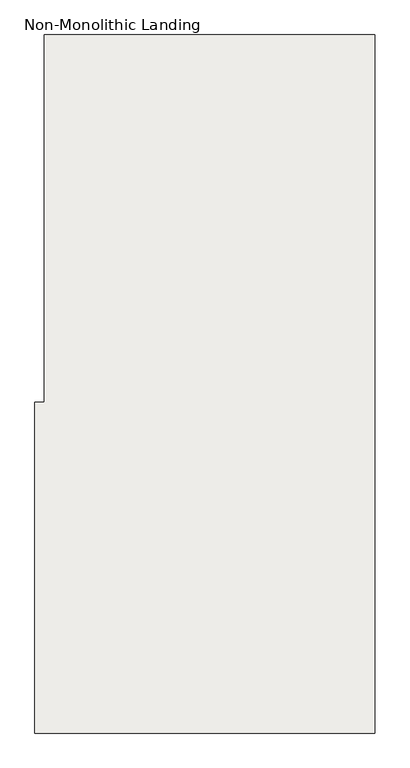
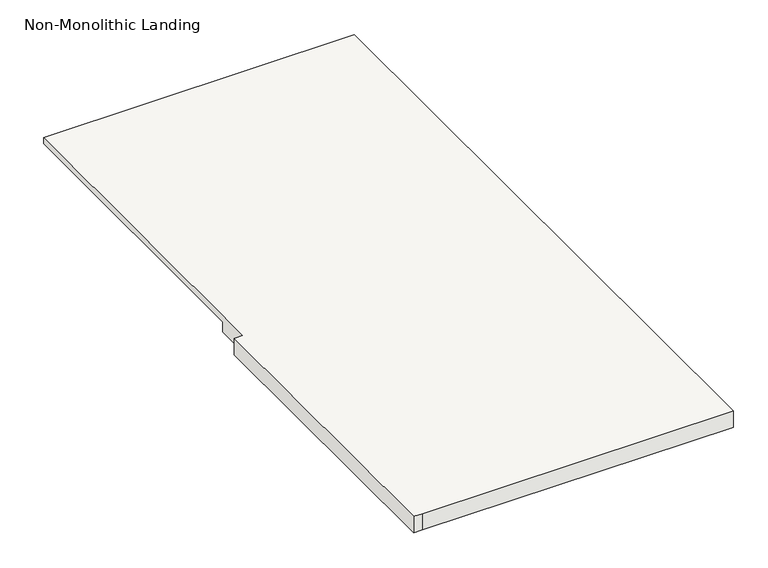
"""IFC4 building model written with IfcOpenShell, lengths in millimetres: slab geometry, Non-Monolithic Landing."""

from ifc_helpers import new_model, si_unit, origin, place, context, project, spatial, faceted_brep, source, transform, mapped, element, save


def non_monolithic_landing_51f18b7d(model_context):
    return source(origin(), model_context, "Body", "Brep", [
        faceted_brep([(923.4845537, -3822.9544725, 1581.15), (948.8845537, -3822.9544725, 1555.75), (948.8845537, -4737.3544725, 1555.75), (923.4845537, -4737.3544725, 1581.15), (923.4845537, -4838.9544725, 1600.2), (898.0845537, -4838.9544725, 1600.2), (898.0845537, -5753.3544725, 1600.2), (923.4845537, -5753.3544725, 1600.2), (1837.8845537, -5753.3544725, 1600.2), (1837.8845537, -3822.9544725, 1600.2), (923.4845537, -3822.9544725, 1600.2), (948.8845537, -4737.3544725, 1549.4), (948.8845537, -3822.9544725, 1549.4), (1837.8845537, -3822.9544725, 1549.4), (1837.8845537, -5753.3544725, 1549.4), (923.4845537, -5753.3544725, 1549.4), (898.0845537, -5753.3544725, 1549.4), (898.0845537, -4838.9544725, 1549.4), (923.4845537, -4838.9544725, 1549.4), (923.4845537, -4737.3544725, 1549.4)], [[[0, 1, 2, 3]], [[4, 5, 6, 7, 8, 9, 10]], [[11, 12, 13, 14, 15, 16, 17, 18, 19]], [[12, 11, 2, 1]], [[11, 19, 3, 2]], [[4, 10, 0, 3, 19, 18]], [[5, 4, 18, 17]], [[6, 5, 17, 16]], [[7, 6, 16, 15]], [[8, 7, 15, 14]], [[9, 8, 14, 13]], [[10, 9, 13, 12, 1, 0]]]),
    ])


if __name__ == "__main__":
    model = new_model("IFC4")
    model_context = context("Model", 3, world=origin())
    ifc_project = project(units=[si_unit("LENGTHUNIT", "METRE", prefix="MILLI")], contexts=[model_context])
    site = spatial("IfcSite", under=ifc_project)
    building = spatial("IfcBuilding", under=site)
    placement = place(None, origin())
    non_monolithic_landing_shape = non_monolithic_landing_51f18b7d(model_context)
    element("IfcSlab", 1, ObjectType="Non-Monolithic Landing", at=placement, inside=building, context=model_context, shape_type="MappedRepresentation", body=[
        mapped(non_monolithic_landing_shape, transform((0.0, 0.0, 0.0), x_axis=(1.0, 0.0, 0.0), y_axis=(0.0, 1.0, 0.0), z_axis=(0.0, 0.0, 1.0))),
    ])
    save(model, "model.ifc")
